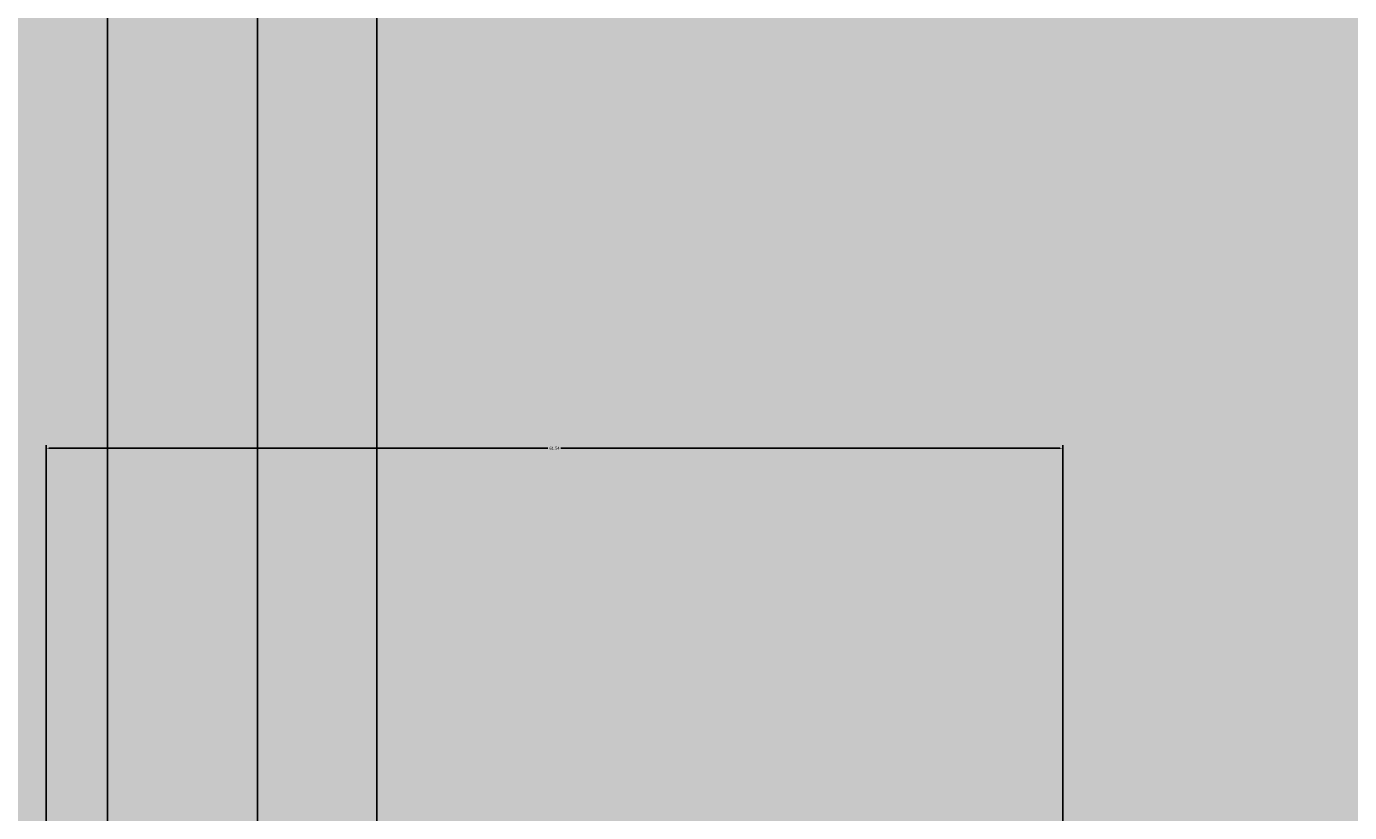
# Model space of a CAD drawing. Units: inches. Extents: x 73 to 607, y 92 to 651.
# Tile 6 of 18: x 368 to 448, y 264 to 311. Entities that reach past the tile are written whole.
import ezdxf

# ---------------------------------------------------------------- set-up
doc = ezdxf.new("R2010")
doc.units = ezdxf.units.IN
doc.header["$MEASUREMENT"] = 0
for name, color, linetype, lineweight in [('A-ANNO-DIMS', 2, 'Continuous', 18), ('A-ELEV-PATT-BKGD', 252, 'Continuous', 13), ('A-ELEV-PATT-SHAD', 8, 'Continuous', 13), ('A-ELEV-PATT-WALL', 254, 'Continuous', 13)]:
    doc.layers.add(name, color=color, linetype=linetype, lineweight=lineweight)
doc.styles.get("Standard").update_dxf_attribs({"font": 'arial.ttf'})
doc.dimstyles.get("Standard").update_dxf_attribs({"dimtxt": 0.18, "dimasz": 0.18, "dimexe": 0.18, "dimexo": 0.0625, "dimgap": 0.09, "dimtad": 0, "dimtih": 1, "dimtoh": 1, "dimdec": 4, "dimzin": 0, "dimdsep": 46, "dimtxsty": 'Standard', "dimcen": 0.09, "dimadec": 0, "dimazin": 0, "dimtfac": 1, "dimtdec": 4, "dimtofl": 0, "dimtmove": 0, "dimatfit": 3, "dimfxl": 1, "dimtolj": 1, "dimtzin": 0, "dimarcsym": 0})

# ---------------------------------------------------------------- blocks, each defined once
blk = doc.blocks.new('*D37')
at = {"layer": 'A-ANNO-DIMS', "color": 0, "lineweight": -2, "transparency": 16777216}
for p, q in [((369.534, 258.754), (369.534, 285.871)), ((369.714, 285.691), (399.908, 285.691)), ((430.89, 285.691), (400.696, 285.691)), ((431.07, 258.754), (431.07, 285.871))]:
    blk.add_line(p, q, dxfattribs=at)
at = {"layer": 'A-ANNO-DIMS', "color": 0, "transparency": 16777216}
for points in [[(369.714, 285.721), (369.714, 285.661), (369.534, 285.691)], [(430.89, 285.721), (430.89, 285.661), (431.07, 285.691)]]:
    blk.add_solid(points, dxfattribs=at)
at = {"layer": 'Defpoints', "color": 0, "transparency": 16777216}
for p in [(431.07, 285.691), (369.534, 258.691), (431.07, 258.691)]:
    blk.add_point(p, dxfattribs=at)
at = {"layer": 'A-ANNO-DIMS', "color": 0, "transparency": 16777216, "insert": (400.302, 285.691), "char_height": 0.18, "attachment_point": 5}
blk.add_mtext('\\A1;61.54', dxfattribs=at)
blk = doc.blocks.new('*D83')
at = {"layer": 'A-ANNO-DIMS', "color": 0, "lineweight": -2, "transparency": 16777216}
for p, q in [((360.849, 238.997), (360.849, 650.981)), ((361.029, 650.801), (366.597, 650.801)), ((373.077, 650.801), (367.508, 650.801)), ((373.257, 231.411), (373.257, 650.981))]:
    blk.add_line(p, q, dxfattribs=at)
at = {"layer": 'A-ANNO-DIMS', "color": 0, "transparency": 16777216}
for points in [[(361.029, 650.831), (361.029, 650.771), (360.849, 650.801)], [(373.077, 650.831), (373.077, 650.771), (373.257, 650.801)]]:
    blk.add_solid(points, dxfattribs=at)
at = {"layer": 'Defpoints', "color": 0, "transparency": 16777216}
for p in [(373.257, 650.801), (360.849, 238.935), (373.257, 231.348)]:
    blk.add_point(p, dxfattribs=at)
at = {"layer": 'A-ANNO-DIMS', "color": 0, "transparency": 16777216, "insert": (367.053, 650.801), "char_height": 0.18, "attachment_point": 5}
blk.add_mtext('\\A1;12.408', dxfattribs=at)
blk = doc.blocks.new('*D84')
at = {"layer": 'A-ANNO-DIMS', "color": 0, "lineweight": -2, "transparency": 16777216}
for p, q in [((373.257, 231.411), (373.257, 650.981)), ((373.437, 650.801), (377.4, 650.801)), ((382.151, 650.801), (378.187, 650.801)), ((382.331, 241.033), (382.331, 650.981))]:
    blk.add_line(p, q, dxfattribs=at)
at = {"layer": 'A-ANNO-DIMS', "color": 0, "transparency": 16777216}
for points in [[(373.437, 650.831), (373.437, 650.771), (373.257, 650.801)], [(382.151, 650.831), (382.151, 650.771), (382.331, 650.801)]]:
    blk.add_solid(points, dxfattribs=at)
at = {"layer": 'Defpoints', "color": 0, "transparency": 16777216}
for p in [(382.331, 650.801), (382.331, 240.97), (373.257, 231.348)]:
    blk.add_point(p, dxfattribs=at)
at = {"layer": 'A-ANNO-DIMS', "color": 0, "transparency": 16777216, "insert": (377.794, 650.801), "char_height": 0.18, "attachment_point": 5}
blk.add_mtext('\\A1;9.074', dxfattribs=at)
blk = doc.blocks.new('*D85')
at = {"layer": 'A-ANNO-DIMS', "color": 0, "lineweight": -2, "transparency": 16777216}
for p, q in [((382.331, 241.033), (382.331, 650.981)), ((382.511, 650.801), (385.55, 650.801)), ((389.373, 650.801), (386.334, 650.801)), ((389.553, 232.521), (389.553, 650.981))]:
    blk.add_line(p, q, dxfattribs=at)
at = {"layer": 'A-ANNO-DIMS', "color": 0, "transparency": 16777216}
for points in [[(382.511, 650.831), (382.511, 650.771), (382.331, 650.801)], [(389.373, 650.831), (389.373, 650.771), (389.553, 650.801)]]:
    blk.add_solid(points, dxfattribs=at)
at = {"layer": 'Defpoints', "color": 0, "transparency": 16777216}
for p in [(389.553, 650.801), (382.331, 240.97), (389.553, 232.458)]:
    blk.add_point(p, dxfattribs=at)
at = {"layer": 'A-ANNO-DIMS', "color": 0, "transparency": 16777216, "insert": (385.942, 650.801), "char_height": 0.18, "attachment_point": 5}
blk.add_mtext('\\A1;7.222', dxfattribs=at)

msp = doc.modelspace()

# ---------------------------------------------------------------- hatches: boundary and pattern name
at = {"layer": 'A-ELEV-PATT-BKGD'}
h = msp.add_hatch(color=256, dxfattribs=at)
h.dxf.hatch_style = 1
h.paths.add_polyline_path([(321.3008, 479.2042), (312.3008, 479.2042), (312.3008, 478.7576), (312.3008, 412.636), (321.3008, 412.636)])
h.paths.add_polyline_path([(312.3008, 504.7576), (256.4726, 504.7576), (256.4726, 503.4576), (312.3008, 503.4576)], flags=17)
h.paths.add_polyline_path([(321.3008, 543.1576), (321.3008, 552.1576), (320.3257, 552.1576), (312.3008, 552.1576), (256.4726, 552.1576), (256.4726, 543.1576), (312.3008, 543.1576), (312.3008, 479.2042), (321.3008, 479.2042)])
h.paths.add_polyline_path([(451.5214, 412.636), (256.4726, 412.636), (256.4726, 403.636), (442.5214, 403.636), (442.5214, 320.2042), (206.1343, 320.2042), (206.1343, 320.9135), (206.1343, 403.636), (256.4726, 403.636), (256.4726, 412.636), (201.6343, 412.636), (201.6343, 320.9135), (201.6343, 320.2042), (201.6343, 311.2042), (256.4726, 311.2042), (451.5214, 311.2042)])
h.paths.add_polyline_path([(431.07, 258.6914), (369.5339, 258.6914), (369.5339, 247.4054), (396.692, 247.4054), (425.07, 247.4054), (425.07, 194.7312), (396.692, 194.6197), (396.692, 194.5366), (369.5339, 194.5366), (369.5339, 185.6619), (431.07, 185.6619)])
h.paths.add_polyline_path([(580.0983, 262.3024), (451.5214, 262.3024), (451.5214, 143.2042), (580.0983, 143.2042)])
h.paths.add_polyline_path([(454.7049, 174.802), (454.7049, 256.6321), (577.9249, 256.6321), (577.9249, 174.802)], flags=16)
h.paths.add_polyline_path([(465.9716, 191.1416, -1), (473.7874, 191.1416, -1)], flags=0)
h.paths.add_polyline_path([(490.5373, 181.6586, -1), (494.9999, 181.6586, -1)], flags=0)
h.paths.add_polyline_path([(476.2996, 209.8287, -1), (500.5844, 209.8287, -1)], flags=0)
h.paths.add_polyline_path([(505.3326, 194.7675, -1), (512.5843, 194.7675, -1)], flags=0)
h.paths.add_polyline_path([(520.9613, 186.679, -1), (526.544, 186.679, -1)], flags=0)
h.paths.add_polyline_path([(466.8103, 225.7267, -1), (470.1573, 225.7267, -1)], flags=0)
h.paths.add_polyline_path([(527.1059, 203.6926, -1), (536.0311, 203.6926, -1)], flags=0)
h.paths.add_polyline_path([(504.775, 232.6995, -1), (513.7002, 232.6995, -1)], flags=0)
h.paths.add_polyline_path([(546.9241, 183.611, -1), (554.7336, 183.611, -1)], flags=0)
h.paths.add_polyline_path([(459.5544, 243.856, -1), (466.8061, 243.856, -1)], flags=0)
h.paths.add_polyline_path([(476.3045, 246.924, -1), (488.5767, 246.924, -1)], flags=0)
h.paths.add_polyline_path([(529.9044, 226.8424, -1), (556.68, 226.8424, -1)], flags=0)
h.paths.add_polyline_path([(554.1814, 203.9716, -1), (561.4331, 203.9716, -1)], flags=0)
h.paths.add_polyline_path([(567.8561, 193.3729, -1), (570.6475, 193.3729, -1)], flags=0)
h.paths.add_polyline_path([(522.3584, 250.271, -1), (525.7053, 250.271, -1)], flags=0)
h.paths.add_polyline_path([(561.9965, 245.2506, -1), (567.5748, 245.2506, -1)], flags=0)
h.paths.add_polyline_path([(347.8686, 194.5366), (341.8686, 194.5366), (341.8686, 194.5452), (314.0144, 194.5452), (314.0144, 188.5452), (347.8686, 188.5452)])
h.paths.add_polyline_path([(347.8686, 253.4054), (314.0144, 253.4054), (314.0144, 247.4054), (341.8686, 247.4054), (347.8686, 247.4054)])
h.paths.add_polyline_path([(304.3559, 253.4054), (298.3559, 253.4054), (298.3559, 188.5452), (304.3559, 188.5452)])
h.paths.add_polyline_path([(450.6603, 552.1576), (369.9727, 552.1576), (369.9727, 479.2042), (374.4727, 479.2042), (374.4727, 547.6576), (446.1603, 547.6576), (446.1603, 479.2042), (450.6603, 479.2042)])
h.paths.add_polyline_path([(374.4727, 479.2042), (369.9727, 479.2042), (369.9727, 465.0632), (374.4727, 465.0632)])
h.paths.add_polyline_path([(450.6603, 479.2042), (446.1603, 479.2042), (446.1603, 465.0632), (450.6603, 465.0632)])
h.paths.add_polyline_path([(256.4726, 281.6039), (109.0983, 281.6039), (100.0983, 281.6039), (100.0983, 167.2042), (100.0983, 143.2042), (109.0983, 143.2042), (109.0983, 167.2042), (109.0983, 272.6039), (256.4726, 272.6039)])
at = {"layer": 'A-ELEV-PATT-SHAD'}
h = msp.add_hatch(color=256, dxfattribs=at)
h.dxf.hatch_style = 1
h.paths.add_polyline_path([(451.5214, 412.636), (256.4726, 412.636), (256.4726, 403.636), (442.5214, 403.636), (442.5214, 320.2042), (206.1343, 320.2042), (206.1343, 320.9135), (206.1343, 403.636), (256.4726, 403.636), (256.4726, 412.636), (201.6343, 412.636), (201.6343, 320.9135), (201.6343, 320.2042), (201.6343, 311.2042), (256.4726, 311.2042), (451.5214, 311.2042)])
h.paths.add_polyline_path([(580.0983, 262.3024), (451.5214, 262.3024), (451.5214, 143.2042), (580.0983, 143.2042)])
h.paths.add_polyline_path([(454.7049, 174.802), (454.7049, 256.6321), (577.9249, 256.6321), (577.9249, 174.802)], flags=16)
h.paths.add_polyline_path([(465.9716, 191.1416, -1), (473.7874, 191.1416, -1)], flags=0)
h.paths.add_polyline_path([(490.5373, 181.6586, -1), (494.9999, 181.6586, -1)], flags=0)
h.paths.add_polyline_path([(476.2996, 209.8287, -1), (500.5844, 209.8287, -1)], flags=0)
h.paths.add_polyline_path([(505.3326, 194.7675, -1), (512.5843, 194.7675, -1)], flags=0)
h.paths.add_polyline_path([(520.9613, 186.679, -1), (526.544, 186.679, -1)], flags=0)
h.paths.add_polyline_path([(466.8103, 225.7267, -1), (470.1573, 225.7267, -1)], flags=0)
h.paths.add_polyline_path([(527.1059, 203.6926, -1), (536.0311, 203.6926, -1)], flags=0)
h.paths.add_polyline_path([(459.5544, 243.856, -1), (466.8061, 243.856, -1)], flags=0)
h.paths.add_polyline_path([(504.775, 232.6995, -1), (513.7002, 232.6995, -1)], flags=0)
h.paths.add_polyline_path([(476.3045, 246.924, -1), (488.5767, 246.924, -1)], flags=0)
h.paths.add_polyline_path([(546.9241, 183.611, -1), (554.7336, 183.611, -1)], flags=0)
h.paths.add_polyline_path([(529.9044, 226.8424, -1), (556.68, 226.8424, -1)], flags=0)
h.paths.add_polyline_path([(554.1814, 203.9716, -1), (561.4331, 203.9716, -1)], flags=0)
h.paths.add_polyline_path([(522.3584, 250.271, -1), (525.7053, 250.271, -1)], flags=0)
h.paths.add_polyline_path([(567.8561, 193.3729, -1), (570.6475, 193.3729, -1)], flags=0)
h.paths.add_polyline_path([(561.9965, 245.2506, -1), (567.5748, 245.2506, -1)], flags=0)
h.paths.add_polyline_path([(431.07, 258.6914), (369.5339, 258.6914), (369.5339, 247.4054), (396.692, 247.4054), (425.07, 247.4054), (425.07, 194.7312), (396.692, 194.6197), (396.692, 194.5366), (369.5339, 194.5366), (369.5339, 185.6619), (431.07, 185.6619)])
h.paths.add_polyline_path([(347.8686, 253.4054), (314.0144, 253.4054), (314.0144, 247.4054), (341.8686, 247.4054), (347.8686, 247.4054)])
h.paths.add_polyline_path([(304.3559, 253.4054), (298.3559, 253.4054), (298.3559, 188.5452), (304.3559, 188.5452)])
h.paths.add_polyline_path([(347.8686, 194.5366), (341.8686, 194.5366), (341.8686, 194.5452), (314.0144, 194.5452), (314.0144, 188.5452), (347.8686, 188.5452)])
at = {"layer": 'A-ELEV-PATT-WALL'}
h = msp.add_hatch(color=256, dxfattribs=at)
h.dxf.hatch_style = 1
h.paths.add_polyline_path([(509.9692, 483.857), (450.6603, 483.857), (450.6603, 465.0632), (446.1603, 465.0632), (446.1603, 484.2142), (374.4727, 484.2142), (374.4727, 465.0632), (369.9727, 465.0632), (369.9727, 484.2142), (321.3008, 484.2142), (321.3008, 412.636), (451.5214, 412.636), (451.5214, 311.2042), (314.0144, 311.2042), (314.0144, 253.4054), (347.8686, 253.4054), (347.8686, 247.4054), (369.5339, 247.4054), (369.5339, 258.6914), (431.07, 258.6914), (431.07, 185.6619), (369.5339, 185.6619), (369.5339, 194.5366), (347.8686, 194.5366), (347.8686, 188.5452), (314.0144, 188.5452), (314.0144, 143.2042), (451.5214, 143.2042), (451.5214, 262.3024), (580.0983, 262.3024), (580.0983, 311.2042), (509.9692, 311.2042)])
h.paths.add_polyline_path([(304.3559, 311.2042), (256.4726, 311.2042), (256.4726, 167.2042), (256.4726, 143.2042), (304.3559, 143.2042), (304.3559, 188.5452), (298.3559, 188.5452), (298.3559, 253.4054), (304.3559, 253.4054)])

# ---------------------------------------------------------------- dimensions: what is measured, and where the dimension line sits
at = {"layer": 'A-ANNO-DIMS'}
for base, p1, p2, override, picture, middle in [((373.2566, 650.801), (360.8489, 238.9349), (373.2566, 231.3482), {"dimdec": 3, "dimlfac": 1, "dimrnd": 0, "dimzin": 0, "dimdsep": 46, "dimlunit": 2}, '*D83', (367.0527, 650.801)), ((382.3308, 650.801), (373.2566, 231.3482), (382.3308, 240.9703), {"dimdec": 3, "dimlfac": 1, "dimrnd": 0, "dimzin": 0, "dimdsep": 46, "dimlunit": 2}, '*D84', (377.7937, 650.801)), ((389.5532, 650.801), (382.3308, 240.9703), (389.5532, 232.4585), {"dimdec": 3, "dimlfac": 1, "dimrnd": 0, "dimzin": 0, "dimdsep": 46, "dimlunit": 2}, '*D85', (385.942, 650.801)), ((431.07, 285.6914), (369.5339, 258.6914), (431.07, 258.6914), {"dimdec": 2, "dimlfac": 1, "dimrnd": 0, "dimzin": 0, "dimdsep": 46, "dimlunit": 2}, '*D37', (400.302, 285.6914))]:
    dim = msp.add_linear_dim(base=base, p1=p1, p2=p2, dimstyle='Standard', override=override, dxfattribs=at)
    dim.commit()
    dim.dimension.update_dxf_attribs({"geometry": picture, "text_midpoint": middle})

doc.saveas('drawing.dxf')
